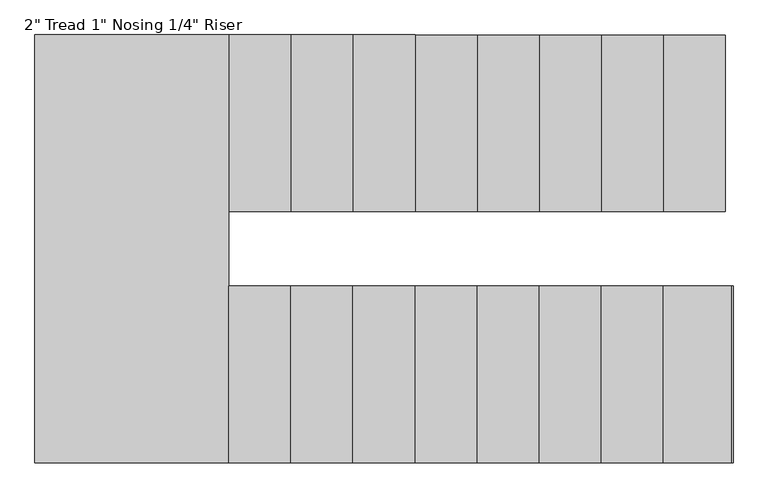
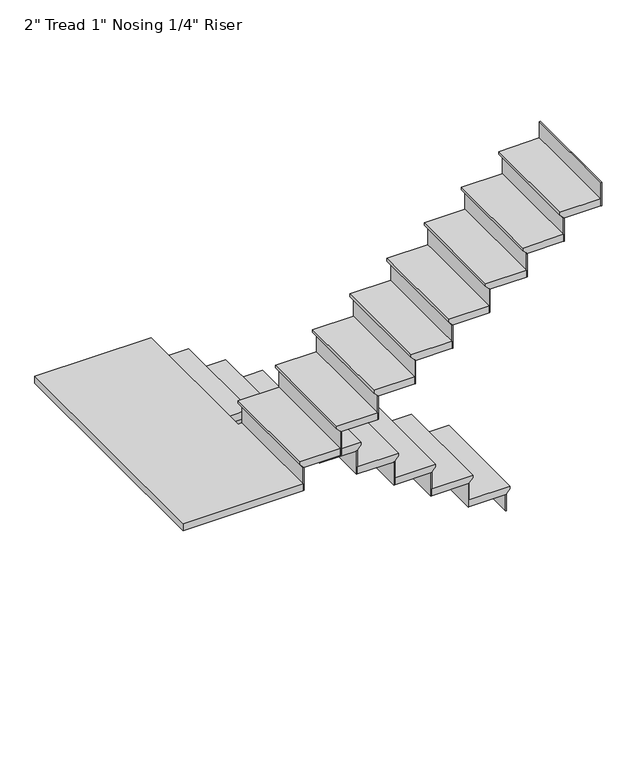
"""IFC4 building model written with IfcOpenShell, lengths in millimetres: stair flight geometry."""

from ifc_helpers import new_model, si_unit, origin, place, context, project, spatial, faceted_brep, source, transform, mapped, element, save


def stair_flight_e970c3af(model_context):
    return source(origin(), model_context, "Body", "Brep", [
        faceted_brep([(-2118.1728655, 1192.5797121, 6244.8722222), (-2118.1728655, 1192.5797121, 6263.9222222), (-2118.1728655, 468.6797121, 6263.9222222), (-2118.1728655, 468.6797121, 6244.8722222), (-2143.5728655, 1192.5797121, 6219.4722222), (-2143.5728655, 468.6797121, 6219.4722222), (-2397.5728655, 1192.5797121, 6263.9222222), (-2397.5728655, 468.6797121, 6263.9222222), (-2143.5728655, 468.6797121, 6213.1222222), (-2397.5728655, 468.6797121, 6213.1222222), (-2397.5728655, 1192.5797121, 6213.1222222), (-2143.5728655, 1192.5797121, 6213.1222222)], [[[0, 1, 2, 3]], [[4, 0, 3, 5]], [[2, 1, 6, 7]], [[8, 9, 10, 11]], [[2, 7, 9, 8, 5, 3]], [[8, 11, 4, 5]], [[6, 1, 0, 4, 11, 10]], [[7, 6, 10, 9]]]),
        faceted_brep([(-2143.5728655, 1192.5797121, 6213.1222222), (-2143.5728655, 1192.5797121, 6096.0), (-2149.9228655, 1192.5797121, 6096.0), (-2149.9228655, 1192.5797121, 6213.1222222), (-2143.5728655, 468.6797121, 6213.1222222), (-2149.9228655, 468.6797121, 6213.1222222), (-2149.9228655, 468.6797121, 6096.0), (-2143.5728655, 468.6797121, 6096.0)], [[[0, 1, 2, 3]], [[4, 5, 6, 7]], [[1, 0, 4, 7]], [[2, 1, 7, 6]], [[3, 2, 6, 5]], [[0, 3, 5, 4]]]),
        faceted_brep([(-2397.5728655, 1192.5797121, 6381.0444444), (-2397.5728655, 1192.5797121, 6213.1222222), (-2403.9228655, 1192.5797121, 6213.1222222), (-2403.9228655, 1192.5797121, 6381.0444444), (-2397.5728655, 468.6797121, 6381.0444444), (-2403.9228655, 468.6797121, 6381.0444444), (-2403.9228655, 468.6797121, 6213.1222222), (-2397.5728655, 468.6797121, 6213.1222222)], [[[0, 1, 2, 3]], [[4, 5, 6, 7]], [[1, 0, 4, 7]], [[2, 1, 7, 6]], [[3, 2, 6, 5]], [[0, 3, 5, 4]]]),
        faceted_brep([(-2372.1728655, 468.6797121, 6431.8444444), (-2372.1728655, 1192.5797121, 6431.8444444), (-2651.5728655, 1192.5797121, 6431.8444444), (-2651.5728655, 468.6797121, 6431.8444444), (-2397.5728655, 468.6797121, 6381.0444444), (-2651.5728655, 468.6797121, 6381.0444444), (-2651.5728655, 1192.5797121, 6381.0444444), (-2397.5728655, 1192.5797121, 6381.0444444), (-2397.5728655, 468.6797121, 6387.3944444), (-2372.1728655, 468.6797121, 6412.7944444), (-2397.5728655, 1192.5797121, 6387.3944444), (-2372.1728655, 1192.5797121, 6412.7944444)], [[[0, 1, 2, 3]], [[4, 5, 6, 7]], [[0, 3, 5, 4, 8, 9]], [[4, 7, 10, 8]], [[2, 1, 11, 10, 7, 6]], [[3, 2, 6, 5]], [[11, 1, 0, 9]], [[10, 11, 9, 8]]]),
        faceted_brep([(-2651.5728655, 1192.5797121, 6548.9666667), (-2651.5728655, 1192.5797121, 6381.0444444), (-2657.9228655, 1192.5797121, 6381.0444444), (-2657.9228655, 1192.5797121, 6548.9666667), (-2651.5728655, 468.6797121, 6548.9666667), (-2657.9228655, 468.6797121, 6548.9666667), (-2657.9228655, 468.6797121, 6381.0444444), (-2651.5728655, 468.6797121, 6381.0444444)], [[[0, 1, 2, 3]], [[4, 5, 6, 7]], [[1, 0, 4, 7]], [[2, 1, 7, 6]], [[3, 2, 6, 5]], [[0, 3, 5, 4]]]),
        faceted_brep([(-2626.1728655, 468.6797121, 6599.7666667), (-2626.1728655, 1192.5797121, 6599.7666667), (-2905.5728655, 1192.5797121, 6599.7666667), (-2905.5728655, 468.6797121, 6599.7666667), (-2651.5728655, 468.6797121, 6548.9666667), (-2905.5728655, 468.6797121, 6548.9666667), (-2905.5728655, 1192.5797121, 6548.9666667), (-2651.5728655, 1192.5797121, 6548.9666667), (-2651.5728655, 468.6797121, 6555.3166667), (-2626.1728655, 468.6797121, 6580.7166667), (-2651.5728655, 1192.5797121, 6555.3166667), (-2626.1728655, 1192.5797121, 6580.7166667)], [[[0, 1, 2, 3]], [[4, 5, 6, 7]], [[0, 3, 5, 4, 8, 9]], [[4, 7, 10, 8]], [[2, 1, 11, 10, 7, 6]], [[3, 2, 6, 5]], [[11, 1, 0, 9]], [[10, 11, 9, 8]]]),
        faceted_brep([(-2905.5728655, 1192.5797121, 6716.8888889), (-2905.5728655, 1192.5797121, 6548.9666667), (-2911.9228655, 1192.5797121, 6548.9666667), (-2911.9228655, 1192.5797121, 6716.8888889), (-2905.5728655, 468.6797121, 6716.8888889), (-2911.9228655, 468.6797121, 6716.8888889), (-2911.9228655, 468.6797121, 6548.9666667), (-2905.5728655, 468.6797121, 6548.9666667)], [[[0, 1, 2, 3]], [[4, 5, 6, 7]], [[1, 0, 4, 7]], [[2, 1, 7, 6]], [[3, 2, 6, 5]], [[0, 3, 5, 4]]]),
        faceted_brep([(-2880.1728655, 468.6797121, 6767.6888889), (-2880.1728655, 1192.5797121, 6767.6888889), (-3159.5728655, 1192.5797121, 6767.6888889), (-3159.5728655, 468.6797121, 6767.6888889), (-2905.5728655, 468.6797121, 6716.8888889), (-3159.5728655, 468.6797121, 6716.8888889), (-3159.5728655, 1192.5797121, 6716.8888889), (-2905.5728655, 1192.5797121, 6716.8888889), (-2905.5728655, 468.6797121, 6723.2388889), (-2880.1728655, 468.6797121, 6748.6388889), (-2905.5728655, 1192.5797121, 6723.2388889), (-2880.1728655, 1192.5797121, 6748.6388889)], [[[0, 1, 2, 3]], [[4, 5, 6, 7]], [[0, 3, 5, 4, 8, 9]], [[4, 7, 10, 8]], [[2, 1, 11, 10, 7, 6]], [[3, 2, 6, 5]], [[11, 1, 0, 9]], [[10, 11, 9, 8]]]),
        faceted_brep([(-3159.5728655, 1192.5797121, 6884.8111111), (-3159.5728655, 1192.5797121, 6716.8888889), (-3165.9228655, 1192.5797121, 6716.8888889), (-3165.9228655, 1192.5797121, 6884.8111111), (-3159.5728655, 468.6797121, 6884.8111111), (-3165.9228655, 468.6797121, 6884.8111111), (-3165.9228655, 468.6797121, 6716.8888889), (-3159.5728655, 468.6797121, 6716.8888889)], [[[0, 1, 2, 3]], [[4, 5, 6, 7]], [[1, 0, 4, 7]], [[2, 1, 7, 6]], [[3, 2, 6, 5]], [[0, 3, 5, 4]]]),
        faceted_brep([(-3134.1728655, 468.6797121, 6935.6111111), (-3134.1728655, 1192.5797121, 6935.6111111), (-3413.5728655, 1192.5797121, 6935.6111111), (-3413.5728655, 468.6797121, 6935.6111111), (-3159.5728655, 468.6797121, 6884.8111111), (-3413.5728655, 468.6797121, 6884.8111111), (-3413.5728655, 1192.5797121, 6884.8111111), (-3159.5728655, 1192.5797121, 6884.8111111), (-3159.5728655, 468.6797121, 6891.1611111), (-3134.1728655, 468.6797121, 6916.5611111), (-3159.5728655, 1192.5797121, 6891.1611111), (-3134.1728655, 1192.5797121, 6916.5611111)], [[[0, 1, 2, 3]], [[4, 5, 6, 7]], [[0, 3, 5, 4, 8, 9]], [[4, 7, 10, 8]], [[2, 1, 11, 10, 7, 6]], [[3, 2, 6, 5]], [[11, 1, 0, 9]], [[10, 11, 9, 8]]]),
        faceted_brep([(-3413.5728655, 1192.5797121, 7052.7333333), (-3413.5728655, 1192.5797121, 6884.8111111), (-3419.9228655, 1192.5797121, 6884.8111111), (-3419.9228655, 1192.5797121, 7052.7333333), (-3413.5728655, 468.6797121, 7052.7333333), (-3419.9228655, 468.6797121, 7052.7333333), (-3419.9228655, 468.6797121, 6884.8111111), (-3413.5728655, 468.6797121, 6884.8111111)], [[[0, 1, 2, 3]], [[4, 5, 6, 7]], [[1, 0, 4, 7]], [[2, 1, 7, 6]], [[3, 2, 6, 5]], [[0, 3, 5, 4]]]),
        faceted_brep([(-3388.1728655, 468.6797121, 7103.5333333), (-3388.1728655, 1192.5797121, 7103.5333333), (-3667.5728655, 1192.5797121, 7103.5333333), (-3667.5728655, 468.6797121, 7103.5333333), (-3413.5728655, 468.6797121, 7052.7333333), (-3667.5728655, 468.6797121, 7052.7333333), (-3667.5728655, 1192.5797121, 7052.7333333), (-3413.5728655, 1192.5797121, 7052.7333333), (-3413.5728655, 468.6797121, 7059.0833333), (-3388.1728655, 468.6797121, 7084.4833333), (-3413.5728655, 1192.5797121, 7059.0833333), (-3388.1728655, 1192.5797121, 7084.4833333)], [[[0, 1, 2, 3]], [[4, 5, 6, 7]], [[0, 3, 5, 4, 8, 9]], [[4, 7, 10, 8]], [[2, 1, 11, 10, 7, 6]], [[3, 2, 6, 5]], [[11, 1, 0, 9]], [[10, 11, 9, 8]]]),
        faceted_brep([(-3667.5728655, 1192.5797121, 7220.6555556), (-3667.5728655, 1192.5797121, 7052.7333333), (-3673.9228655, 1192.5797121, 7052.7333333), (-3673.9228655, 1192.5797121, 7220.6555556), (-3667.5728655, 468.6797121, 7220.6555556), (-3673.9228655, 468.6797121, 7220.6555556), (-3673.9228655, 468.6797121, 7052.7333333), (-3667.5728655, 468.6797121, 7052.7333333)], [[[0, 1, 2, 3]], [[4, 5, 6, 7]], [[1, 0, 4, 7]], [[2, 1, 7, 6]], [[3, 2, 6, 5]], [[0, 3, 5, 4]]]),
        faceted_brep([(-3642.1728655, 468.6797121, 7271.4555556), (-3642.1728655, 1192.5797121, 7271.4555556), (-3921.5728655, 1192.5797121, 7271.4555556), (-3921.5728655, 468.6797121, 7271.4555556), (-3667.5728655, 468.6797121, 7220.6555556), (-3921.5728655, 468.6797121, 7220.6555556), (-3921.5728655, 1192.5797121, 7220.6555556), (-3667.5728655, 1192.5797121, 7220.6555556), (-3667.5728655, 468.6797121, 7227.0055556), (-3642.1728655, 468.6797121, 7252.4055556), (-3667.5728655, 1192.5797121, 7227.0055556), (-3642.1728655, 1192.5797121, 7252.4055556)], [[[0, 1, 2, 3]], [[4, 5, 6, 7]], [[0, 3, 5, 4, 8, 9]], [[4, 7, 10, 8]], [[2, 1, 11, 10, 7, 6]], [[3, 2, 6, 5]], [[11, 1, 0, 9]], [[10, 11, 9, 8]]]),
        faceted_brep([(-3921.5728655, 1192.5797121, 7388.5777778), (-3921.5728655, 1192.5797121, 7220.6555556), (-3927.9228655, 1192.5797121, 7220.6555556), (-3927.9228655, 1192.5797121, 7388.5777778), (-3921.5728655, 468.6797121, 7388.5777778), (-3927.9228655, 468.6797121, 7388.5777778), (-3927.9228655, 468.6797121, 7220.6555556), (-3921.5728655, 468.6797121, 7220.6555556)], [[[0, 1, 2, 3]], [[4, 5, 6, 7]], [[1, 0, 4, 7]], [[2, 1, 7, 6]], [[3, 2, 6, 5]], [[0, 3, 5, 4]]]),
        faceted_brep([(-3896.1728655, 468.6797121, 7439.3777778), (-3896.1728655, 1192.5797121, 7439.3777778), (-4175.5728655, 1192.5797121, 7439.3777778), (-4175.5728655, 468.6797121, 7439.3777778), (-3921.5728655, 468.6797121, 7388.5777778), (-4175.5728655, 468.6797121, 7388.5777778), (-4175.5728655, 1192.5797121, 7388.5777778), (-3921.5728655, 1192.5797121, 7388.5777778), (-3921.5728655, 468.6797121, 7394.9277778), (-3896.1728655, 468.6797121, 7420.3277778), (-3921.5728655, 1192.5797121, 7394.9277778), (-3896.1728655, 1192.5797121, 7420.3277778)], [[[0, 1, 2, 3]], [[4, 5, 6, 7]], [[0, 3, 5, 4, 8, 9]], [[4, 7, 10, 8]], [[2, 1, 11, 10, 7, 6]], [[3, 2, 6, 5]], [[11, 1, 0, 9]], [[10, 11, 9, 8]]]),
        faceted_brep([(-4175.5728655, 1192.5797121, 7556.5), (-4175.5728655, 1192.5797121, 7388.5777778), (-4181.9228655, 1192.5797121, 7388.5777778), (-4181.9228655, 1192.5797121, 7556.5), (-4175.5728655, 468.6797121, 7556.5), (-4181.9228655, 468.6797121, 7556.5), (-4181.9228655, 468.6797121, 7388.5777778), (-4175.5728655, 468.6797121, 7388.5777778)], [[[0, 1, 2, 3]], [[4, 5, 6, 7]], [[1, 0, 4, 7]], [[2, 1, 7, 6]], [[3, 2, 6, 5]], [[0, 3, 5, 4]]]),
        faceted_brep([(-4124.7728655, 163.8797121, 7607.3), (-4150.1728655, 163.8797121, 7607.3), (-4150.1728655, 1192.5797121, 7607.3), (-4943.9394105, 1192.5797121, 7607.3), (-4943.9394105, -560.0202879, 7607.3), (-4124.7728655, -560.0202879, 7607.3), (-4150.1728655, 163.8797121, 7556.5), (-4124.7728655, 163.8797121, 7556.5), (-4124.7728655, -560.0202879, 7556.5), (-4943.9394105, -560.0202879, 7556.5), (-4943.9394105, 1192.5797121, 7556.5), (-4175.5728655, 1192.5797121, 7556.5), (-4175.5728655, 468.6797121, 7556.5), (-4150.1728655, 468.6797121, 7556.5), (-4150.1728655, 468.6797121, 7588.25), (-4150.1728655, 1192.5797121, 7588.25), (-4175.5728655, 468.6797121, 7562.85), (-4175.5728655, 1192.5797121, 7562.85)], [[[0, 1, 2, 3, 4, 5]], [[6, 7, 8, 9, 10, 11, 12, 13]], [[1, 0, 7, 6]], [[2, 1, 6, 13, 14, 15]], [[13, 12, 16, 14]], [[12, 11, 17, 16]], [[3, 2, 15, 17, 11, 10]], [[4, 3, 10, 9]], [[5, 4, 9, 8]], [[0, 5, 8, 7]], [[17, 15, 14, 16]]]),
        faceted_brep([(-4124.7728655, -560.0202879, 7724.4222222), (-4124.7728655, -560.0202879, 7556.5), (-4118.4228655, -560.0202879, 7556.5), (-4118.4228655, -560.0202879, 7724.4222222), (-4124.7728655, 163.8797121, 7724.4222222), (-4118.4228655, 163.8797121, 7724.4222222), (-4118.4228655, 163.8797121, 7556.5), (-4124.7728655, 163.8797121, 7556.5)], [[[0, 1, 2, 3]], [[4, 5, 6, 7]], [[1, 0, 4, 7]], [[2, 1, 7, 6]], [[3, 2, 6, 5]], [[0, 3, 5, 4]]]),
        faceted_brep([(-4150.1728655, 163.8797121, 7775.2222222), (-4150.1728655, -560.0202879, 7775.2222222), (-3870.7728655, -560.0202879, 7775.2222222), (-3870.7728655, 163.8797121, 7775.2222222), (-4124.7728655, 163.8797121, 7724.4222222), (-3870.7728655, 163.8797121, 7724.4222222), (-3870.7728655, -560.0202879, 7724.4222222), (-4124.7728655, -560.0202879, 7724.4222222), (-4124.7728655, 163.8797121, 7730.7722222), (-4150.1728655, 163.8797121, 7756.1722222), (-4124.7728655, -560.0202879, 7730.7722222), (-4150.1728655, -560.0202879, 7756.1722222)], [[[0, 1, 2, 3]], [[4, 5, 6, 7]], [[0, 3, 5, 4, 8, 9]], [[4, 7, 10, 8]], [[2, 1, 11, 10, 7, 6]], [[3, 2, 6, 5]], [[11, 1, 0, 9]], [[10, 11, 9, 8]]]),
        faceted_brep([(-3870.7728655, -560.0202879, 7892.3444444), (-3870.7728655, -560.0202879, 7724.4222222), (-3864.4228655, -560.0202879, 7724.4222222), (-3864.4228655, -560.0202879, 7892.3444444), (-3870.7728655, 163.8797121, 7892.3444444), (-3864.4228655, 163.8797121, 7892.3444444), (-3864.4228655, 163.8797121, 7724.4222222), (-3870.7728655, 163.8797121, 7724.4222222)], [[[0, 1, 2, 3]], [[4, 5, 6, 7]], [[1, 0, 4, 7]], [[2, 1, 7, 6]], [[3, 2, 6, 5]], [[0, 3, 5, 4]]]),
        faceted_brep([(-3896.1728655, 163.8797121, 7943.1444444), (-3896.1728655, -560.0202879, 7943.1444444), (-3616.7728655, -560.0202879, 7943.1444444), (-3616.7728655, 163.8797121, 7943.1444444), (-3870.7728655, 163.8797121, 7892.3444444), (-3616.7728655, 163.8797121, 7892.3444444), (-3616.7728655, -560.0202879, 7892.3444444), (-3870.7728655, -560.0202879, 7892.3444444), (-3870.7728655, 163.8797121, 7898.6944444), (-3896.1728655, 163.8797121, 7924.0944444), (-3870.7728655, -560.0202879, 7898.6944444), (-3896.1728655, -560.0202879, 7924.0944444)], [[[0, 1, 2, 3]], [[4, 5, 6, 7]], [[0, 3, 5, 4, 8, 9]], [[4, 7, 10, 8]], [[2, 1, 11, 10, 7, 6]], [[3, 2, 6, 5]], [[11, 1, 0, 9]], [[10, 11, 9, 8]]]),
        faceted_brep([(-3616.7728655, -560.0202879, 8060.2666667), (-3616.7728655, -560.0202879, 7892.3444444), (-3610.4228655, -560.0202879, 7892.3444444), (-3610.4228655, -560.0202879, 8060.2666667), (-3616.7728655, 163.8797121, 8060.2666667), (-3610.4228655, 163.8797121, 8060.2666667), (-3610.4228655, 163.8797121, 7892.3444444), (-3616.7728655, 163.8797121, 7892.3444444)], [[[0, 1, 2, 3]], [[4, 5, 6, 7]], [[1, 0, 4, 7]], [[2, 1, 7, 6]], [[3, 2, 6, 5]], [[0, 3, 5, 4]]]),
        faceted_brep([(-3642.1728655, 163.8797121, 8111.0666667), (-3642.1728655, -560.0202879, 8111.0666667), (-3362.7728655, -560.0202879, 8111.0666667), (-3362.7728655, 163.8797121, 8111.0666667), (-3616.7728655, 163.8797121, 8060.2666667), (-3362.7728655, 163.8797121, 8060.2666667), (-3362.7728655, -560.0202879, 8060.2666667), (-3616.7728655, -560.0202879, 8060.2666667), (-3616.7728655, 163.8797121, 8066.6166667), (-3642.1728655, 163.8797121, 8092.0166667), (-3616.7728655, -560.0202879, 8066.6166667), (-3642.1728655, -560.0202879, 8092.0166667)], [[[0, 1, 2, 3]], [[4, 5, 6, 7]], [[0, 3, 5, 4, 8, 9]], [[4, 7, 10, 8]], [[2, 1, 11, 10, 7, 6]], [[3, 2, 6, 5]], [[11, 1, 0, 9]], [[10, 11, 9, 8]]]),
        faceted_brep([(-3362.7728655, -560.0202879, 8228.1888889), (-3362.7728655, -560.0202879, 8060.2666667), (-3356.4228655, -560.0202879, 8060.2666667), (-3356.4228655, -560.0202879, 8228.1888889), (-3362.7728655, 163.8797121, 8228.1888889), (-3356.4228655, 163.8797121, 8228.1888889), (-3356.4228655, 163.8797121, 8060.2666667), (-3362.7728655, 163.8797121, 8060.2666667)], [[[0, 1, 2, 3]], [[4, 5, 6, 7]], [[1, 0, 4, 7]], [[2, 1, 7, 6]], [[3, 2, 6, 5]], [[0, 3, 5, 4]]]),
        faceted_brep([(-3388.1728655, 163.8797121, 8278.9888889), (-3388.1728655, -560.0202879, 8278.9888889), (-3108.7728655, -560.0202879, 8278.9888889), (-3108.7728655, 163.8797121, 8278.9888889), (-3362.7728655, 163.8797121, 8228.1888889), (-3108.7728655, 163.8797121, 8228.1888889), (-3108.7728655, -560.0202879, 8228.1888889), (-3362.7728655, -560.0202879, 8228.1888889), (-3362.7728655, 163.8797121, 8234.5388889), (-3388.1728655, 163.8797121, 8259.9388889), (-3362.7728655, -560.0202879, 8234.5388889), (-3388.1728655, -560.0202879, 8259.9388889)], [[[0, 1, 2, 3]], [[4, 5, 6, 7]], [[0, 3, 5, 4, 8, 9]], [[4, 7, 10, 8]], [[2, 1, 11, 10, 7, 6]], [[3, 2, 6, 5]], [[11, 1, 0, 9]], [[10, 11, 9, 8]]]),
        faceted_brep([(-3108.7728655, -560.0202879, 8396.1111111), (-3108.7728655, -560.0202879, 8228.1888889), (-3102.4228655, -560.0202879, 8228.1888889), (-3102.4228655, -560.0202879, 8396.1111111), (-3108.7728655, 163.8797121, 8396.1111111), (-3102.4228655, 163.8797121, 8396.1111111), (-3102.4228655, 163.8797121, 8228.1888889), (-3108.7728655, 163.8797121, 8228.1888889)], [[[0, 1, 2, 3]], [[4, 5, 6, 7]], [[1, 0, 4, 7]], [[2, 1, 7, 6]], [[3, 2, 6, 5]], [[0, 3, 5, 4]]]),
        faceted_brep([(-3134.1728655, 163.8797121, 8446.9111111), (-3134.1728655, -560.0202879, 8446.9111111), (-2854.7728655, -560.0202879, 8446.9111111), (-2854.7728655, 163.8797121, 8446.9111111), (-3108.7728655, 163.8797121, 8396.1111111), (-2854.7728655, 163.8797121, 8396.1111111), (-2854.7728655, -560.0202879, 8396.1111111), (-3108.7728655, -560.0202879, 8396.1111111), (-3108.7728655, 163.8797121, 8402.4611111), (-3134.1728655, 163.8797121, 8427.8611111), (-3108.7728655, -560.0202879, 8402.4611111), (-3134.1728655, -560.0202879, 8427.8611111)], [[[0, 1, 2, 3]], [[4, 5, 6, 7]], [[0, 3, 5, 4, 8, 9]], [[4, 7, 10, 8]], [[2, 1, 11, 10, 7, 6]], [[3, 2, 6, 5]], [[11, 1, 0, 9]], [[10, 11, 9, 8]]]),
        faceted_brep([(-2854.7728655, -560.0202879, 8564.0333333), (-2854.7728655, -560.0202879, 8396.1111111), (-2848.4228655, -560.0202879, 8396.1111111), (-2848.4228655, -560.0202879, 8564.0333333), (-2854.7728655, 163.8797121, 8564.0333333), (-2848.4228655, 163.8797121, 8564.0333333), (-2848.4228655, 163.8797121, 8396.1111111), (-2854.7728655, 163.8797121, 8396.1111111)], [[[0, 1, 2, 3]], [[4, 5, 6, 7]], [[1, 0, 4, 7]], [[2, 1, 7, 6]], [[3, 2, 6, 5]], [[0, 3, 5, 4]]]),
        faceted_brep([(-2880.1728655, 163.8797121, 8614.8333333), (-2880.1728655, -560.0202879, 8614.8333333), (-2600.7728655, -560.0202879, 8614.8333333), (-2600.7728655, 163.8797121, 8614.8333333), (-2854.7728655, 163.8797121, 8564.0333333), (-2600.7728655, 163.8797121, 8564.0333333), (-2600.7728655, -560.0202879, 8564.0333333), (-2854.7728655, -560.0202879, 8564.0333333), (-2854.7728655, 163.8797121, 8570.3833333), (-2880.1728655, 163.8797121, 8595.7833333), (-2854.7728655, -560.0202879, 8570.3833333), (-2880.1728655, -560.0202879, 8595.7833333)], [[[0, 1, 2, 3]], [[4, 5, 6, 7]], [[0, 3, 5, 4, 8, 9]], [[4, 7, 10, 8]], [[2, 1, 11, 10, 7, 6]], [[3, 2, 6, 5]], [[11, 1, 0, 9]], [[10, 11, 9, 8]]]),
        faceted_brep([(-2600.7728655, -560.0202879, 8731.9555556), (-2600.7728655, -560.0202879, 8564.0333333), (-2594.4228655, -560.0202879, 8564.0333333), (-2594.4228655, -560.0202879, 8731.9555556), (-2600.7728655, 163.8797121, 8731.9555556), (-2594.4228655, 163.8797121, 8731.9555556), (-2594.4228655, 163.8797121, 8564.0333333), (-2600.7728655, 163.8797121, 8564.0333333)], [[[0, 1, 2, 3]], [[4, 5, 6, 7]], [[1, 0, 4, 7]], [[2, 1, 7, 6]], [[3, 2, 6, 5]], [[0, 3, 5, 4]]]),
        faceted_brep([(-2626.1728655, 163.8797121, 8782.7555556), (-2626.1728655, -560.0202879, 8782.7555556), (-2346.7728655, -560.0202879, 8782.7555556), (-2346.7728655, 163.8797121, 8782.7555556), (-2600.7728655, 163.8797121, 8731.9555556), (-2346.7728655, 163.8797121, 8731.9555556), (-2346.7728655, -560.0202879, 8731.9555556), (-2600.7728655, -560.0202879, 8731.9555556), (-2600.7728655, 163.8797121, 8738.3055556), (-2626.1728655, 163.8797121, 8763.7055556), (-2600.7728655, -560.0202879, 8738.3055556), (-2626.1728655, -560.0202879, 8763.7055556)], [[[0, 1, 2, 3]], [[4, 5, 6, 7]], [[0, 3, 5, 4, 8, 9]], [[4, 7, 10, 8]], [[2, 1, 11, 10, 7, 6]], [[3, 2, 6, 5]], [[11, 1, 0, 9]], [[10, 11, 9, 8]]]),
        faceted_brep([(-2346.7728655, -560.0202879, 8899.8777778), (-2346.7728655, -560.0202879, 8731.9555556), (-2340.4228655, -560.0202879, 8731.9555556), (-2340.4228655, -560.0202879, 8899.8777778), (-2346.7728655, 163.8797121, 8899.8777778), (-2340.4228655, 163.8797121, 8899.8777778), (-2340.4228655, 163.8797121, 8731.9555556), (-2346.7728655, 163.8797121, 8731.9555556)], [[[0, 1, 2, 3]], [[4, 5, 6, 7]], [[1, 0, 4, 7]], [[2, 1, 7, 6]], [[3, 2, 6, 5]], [[0, 3, 5, 4]]]),
        faceted_brep([(-2092.7728655, -560.0202879, 9067.8), (-2092.7728655, -560.0202879, 8899.8777778), (-2086.4228655, -560.0202879, 8899.8777778), (-2086.4228655, -560.0202879, 9067.8), (-2092.7728655, 163.8797121, 9067.8), (-2086.4228655, 163.8797121, 9067.8), (-2086.4228655, 163.8797121, 8899.8777778), (-2092.7728655, 163.8797121, 8899.8777778)], [[[0, 1, 2, 3]], [[4, 5, 6, 7]], [[1, 0, 4, 7]], [[2, 1, 7, 6]], [[3, 2, 6, 5]], [[0, 3, 5, 4]]]),
        faceted_brep([(-2372.1728655, 163.8797121, 8950.6777778), (-2372.1728655, -560.0202879, 8950.6777778), (-2092.7728655, -560.0202879, 8950.6777778), (-2092.7728655, 163.8797121, 8950.6777778), (-2346.7728655, 163.8797121, 8899.8777778), (-2092.7728655, 163.8797121, 8899.8777778), (-2092.7728655, -560.0202879, 8899.8777778), (-2346.7728655, -560.0202879, 8899.8777778), (-2346.7728655, 163.8797121, 8906.2277778), (-2372.1728655, 163.8797121, 8931.6277778), (-2346.7728655, -560.0202879, 8906.2277778), (-2372.1728655, -560.0202879, 8931.6277778)], [[[0, 1, 2, 3]], [[4, 5, 6, 7]], [[0, 3, 5, 4, 8, 9]], [[4, 7, 10, 8]], [[2, 1, 11, 10, 7, 6]], [[3, 2, 6, 5]], [[11, 1, 0, 9]], [[10, 11, 9, 8]]]),
    ])


if __name__ == "__main__":
    model = new_model("IFC4")
    model_context = context("Model", 3, world=origin())
    ifc_project = project(units=[si_unit("LENGTHUNIT", "METRE", prefix="MILLI")], contexts=[model_context])
    site = spatial("IfcSite", under=ifc_project)
    building = spatial("IfcBuilding", under=site)
    placement = place(None, origin())
    stair_flight_shape = stair_flight_e970c3af(model_context)
    element("IfcStairFlight", 1, ObjectType="2\" Tread 1\" Nosing 1/4\" Riser", at=placement, inside=building, context=model_context, shape_type="MappedRepresentation", body=[
        mapped(stair_flight_shape, transform((0.0, 0.0, 0.0), x_axis=(1.0, 0.0, 0.0), y_axis=(0.0, 1.0, 0.0), z_axis=(0.0, 0.0, 1.0))),
    ])
    save(model, "model.ifc")
